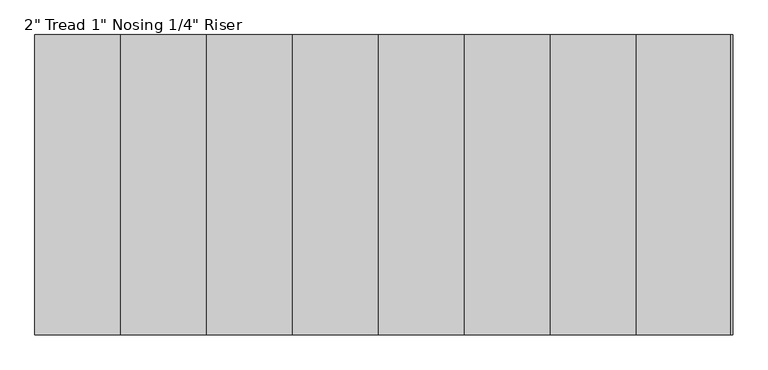
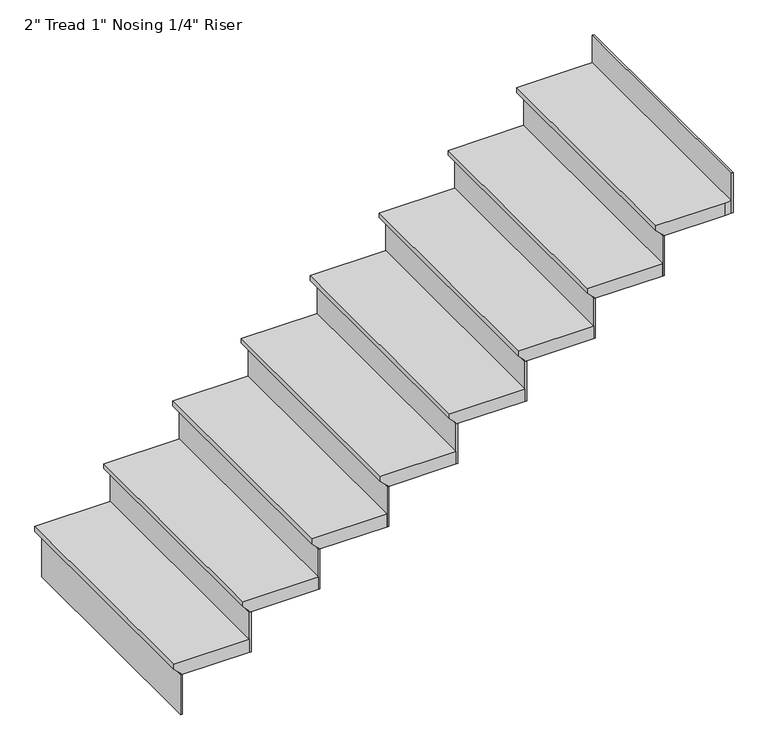
"""IFC4 building model written with IfcOpenShell, lengths in millimetres: stair flight geometry."""

from ifc_helpers import new_model, si_unit, origin, place, context, project, spatial, faceted_brep, source, transform, mapped, element, save


def stair_flight_55fbbb17(model_context):
    return source(origin(), model_context, "Body", "Brep", [
        faceted_brep([(-13886.5772527, 10889.0453953, 943.4763158), (-13886.5772527, 10889.0453953, 962.5263158), (-13886.5772527, 11803.4453953, 962.5263158), (-13886.5772527, 11803.4453953, 943.4763158), (-13861.1772527, 10889.0453953, 918.0763158), (-13861.1772527, 11803.4453953, 918.0763158), (-13599.537409, 10889.0453953, 962.5263158), (-13599.537409, 11803.4453953, 962.5263158), (-13861.1772527, 11803.4453953, 911.7263158), (-13599.537409, 11803.4453953, 911.7263158), (-13599.537409, 10889.0453953, 911.7263158), (-13861.1772527, 10889.0453953, 911.7263158)], [[[0, 1, 2, 3]], [[4, 0, 3, 5]], [[2, 1, 6, 7]], [[8, 9, 10, 11]], [[2, 7, 9, 8, 5, 3]], [[8, 11, 4, 5]], [[6, 1, 0, 4, 11, 10]], [[7, 6, 10, 9]]]),
        faceted_brep([(-13861.1772527, 10889.0453953, 911.7263158), (-13861.1772527, 10889.0453953, 751.3052632), (-13854.8272527, 10889.0453953, 751.3052632), (-13854.8272527, 10889.0453953, 911.7263158), (-13861.1772527, 11803.4453953, 911.7263158), (-13854.8272527, 11803.4453953, 911.7263158), (-13854.8272527, 11803.4453953, 751.3052632), (-13861.1772527, 11803.4453953, 751.3052632)], [[[0, 1, 2, 3]], [[4, 5, 6, 7]], [[1, 0, 4, 7]], [[2, 1, 7, 6]], [[3, 2, 6, 5]], [[0, 3, 5, 4]]]),
        faceted_brep([(-13599.537409, 10889.0453953, 1072.1473684), (-13599.537409, 10889.0453953, 911.7263158), (-13593.187409, 10889.0453953, 911.7263158), (-13593.187409, 10889.0453953, 1072.1473684), (-13599.537409, 11803.4453953, 1072.1473684), (-13593.187409, 11803.4453953, 1072.1473684), (-13593.187409, 11803.4453953, 911.7263158), (-13599.537409, 11803.4453953, 911.7263158)], [[[0, 1, 2, 3]], [[4, 5, 6, 7]], [[1, 0, 4, 7]], [[2, 1, 7, 6]], [[3, 2, 6, 5]], [[0, 3, 5, 4]]]),
        faceted_brep([(-13624.937409, 11803.4453953, 1122.9473684), (-13624.937409, 10889.0453953, 1122.9473684), (-13337.8975652, 10889.0453953, 1122.9473684), (-13337.8975652, 11803.4453953, 1122.9473684), (-13599.537409, 11803.4453953, 1072.1473684), (-13337.8975652, 11803.4453953, 1072.1473684), (-13337.8975652, 10889.0453953, 1072.1473684), (-13599.537409, 10889.0453953, 1072.1473684), (-13599.537409, 11803.4453953, 1078.4973684), (-13624.937409, 11803.4453953, 1103.8973684), (-13599.537409, 10889.0453953, 1078.4973684), (-13624.937409, 10889.0453953, 1103.8973684)], [[[0, 1, 2, 3]], [[4, 5, 6, 7]], [[0, 3, 5, 4, 8, 9]], [[4, 7, 10, 8]], [[2, 1, 11, 10, 7, 6]], [[3, 2, 6, 5]], [[11, 1, 0, 9]], [[10, 11, 9, 8]]]),
        faceted_brep([(-13337.8975652, 10889.0453953, 1232.5684211), (-13337.8975652, 10889.0453953, 1072.1473684), (-13331.5475652, 10889.0453953, 1072.1473684), (-13331.5475652, 10889.0453953, 1232.5684211), (-13337.8975652, 11803.4453953, 1232.5684211), (-13331.5475652, 11803.4453953, 1232.5684211), (-13331.5475652, 11803.4453953, 1072.1473684), (-13337.8975652, 11803.4453953, 1072.1473684)], [[[0, 1, 2, 3]], [[4, 5, 6, 7]], [[1, 0, 4, 7]], [[2, 1, 7, 6]], [[3, 2, 6, 5]], [[0, 3, 5, 4]]]),
        faceted_brep([(-13363.2975652, 11803.4453953, 1283.3684211), (-13363.2975652, 10889.0453953, 1283.3684211), (-13076.2577215, 10889.0453953, 1283.3684211), (-13076.2577215, 11803.4453953, 1283.3684211), (-13337.8975652, 11803.4453953, 1232.5684211), (-13076.2577215, 11803.4453953, 1232.5684211), (-13076.2577215, 10889.0453953, 1232.5684211), (-13337.8975652, 10889.0453953, 1232.5684211), (-13337.8975652, 11803.4453953, 1238.9184211), (-13363.2975652, 11803.4453953, 1264.3184211), (-13337.8975652, 10889.0453953, 1238.9184211), (-13363.2975652, 10889.0453953, 1264.3184211)], [[[0, 1, 2, 3]], [[4, 5, 6, 7]], [[0, 3, 5, 4, 8, 9]], [[4, 7, 10, 8]], [[2, 1, 11, 10, 7, 6]], [[3, 2, 6, 5]], [[11, 1, 0, 9]], [[10, 11, 9, 8]]]),
        faceted_brep([(-13076.2577215, 10889.0453953, 1392.9894737), (-13076.2577215, 10889.0453953, 1232.5684211), (-13069.9077215, 10889.0453953, 1232.5684211), (-13069.9077215, 10889.0453953, 1392.9894737), (-13076.2577215, 11803.4453953, 1392.9894737), (-13069.9077215, 11803.4453953, 1392.9894737), (-13069.9077215, 11803.4453953, 1232.5684211), (-13076.2577215, 11803.4453953, 1232.5684211)], [[[0, 1, 2, 3]], [[4, 5, 6, 7]], [[1, 0, 4, 7]], [[2, 1, 7, 6]], [[3, 2, 6, 5]], [[0, 3, 5, 4]]]),
        faceted_brep([(-13101.6577215, 11803.4453953, 1443.7894737), (-13101.6577215, 10889.0453953, 1443.7894737), (-12814.6178777, 10889.0453953, 1443.7894737), (-12814.6178777, 11803.4453953, 1443.7894737), (-13076.2577215, 11803.4453953, 1392.9894737), (-12814.6178777, 11803.4453953, 1392.9894737), (-12814.6178777, 10889.0453953, 1392.9894737), (-13076.2577215, 10889.0453953, 1392.9894737), (-13076.2577215, 11803.4453953, 1399.3394737), (-13101.6577215, 11803.4453953, 1424.7394737), (-13076.2577215, 10889.0453953, 1399.3394737), (-13101.6577215, 10889.0453953, 1424.7394737)], [[[0, 1, 2, 3]], [[4, 5, 6, 7]], [[0, 3, 5, 4, 8, 9]], [[4, 7, 10, 8]], [[2, 1, 11, 10, 7, 6]], [[3, 2, 6, 5]], [[11, 1, 0, 9]], [[10, 11, 9, 8]]]),
        faceted_brep([(-12814.6178777, 10889.0453953, 1553.4105263), (-12814.6178777, 10889.0453953, 1392.9894737), (-12808.2678777, 10889.0453953, 1392.9894737), (-12808.2678777, 10889.0453953, 1553.4105263), (-12814.6178777, 11803.4453953, 1553.4105263), (-12808.2678777, 11803.4453953, 1553.4105263), (-12808.2678777, 11803.4453953, 1392.9894737), (-12814.6178777, 11803.4453953, 1392.9894737)], [[[0, 1, 2, 3]], [[4, 5, 6, 7]], [[1, 0, 4, 7]], [[2, 1, 7, 6]], [[3, 2, 6, 5]], [[0, 3, 5, 4]]]),
        faceted_brep([(-12840.0178777, 11803.4453953, 1604.2105263), (-12840.0178777, 10889.0453953, 1604.2105263), (-12552.978034, 10889.0453953, 1604.2105263), (-12552.978034, 11803.4453953, 1604.2105263), (-12814.6178777, 11803.4453953, 1553.4105263), (-12552.978034, 11803.4453953, 1553.4105263), (-12552.978034, 10889.0453953, 1553.4105263), (-12814.6178777, 10889.0453953, 1553.4105263), (-12814.6178777, 11803.4453953, 1559.7605263), (-12840.0178777, 11803.4453953, 1585.1605263), (-12814.6178777, 10889.0453953, 1559.7605263), (-12840.0178777, 10889.0453953, 1585.1605263)], [[[0, 1, 2, 3]], [[4, 5, 6, 7]], [[0, 3, 5, 4, 8, 9]], [[4, 7, 10, 8]], [[2, 1, 11, 10, 7, 6]], [[3, 2, 6, 5]], [[11, 1, 0, 9]], [[10, 11, 9, 8]]]),
        faceted_brep([(-12552.978034, 10889.0453953, 1713.8315789), (-12552.978034, 10889.0453953, 1553.4105263), (-12546.628034, 10889.0453953, 1553.4105263), (-12546.628034, 10889.0453953, 1713.8315789), (-12552.978034, 11803.4453953, 1713.8315789), (-12546.628034, 11803.4453953, 1713.8315789), (-12546.628034, 11803.4453953, 1553.4105263), (-12552.978034, 11803.4453953, 1553.4105263)], [[[0, 1, 2, 3]], [[4, 5, 6, 7]], [[1, 0, 4, 7]], [[2, 1, 7, 6]], [[3, 2, 6, 5]], [[0, 3, 5, 4]]]),
        faceted_brep([(-12578.378034, 11803.4453953, 1764.6315789), (-12578.378034, 10889.0453953, 1764.6315789), (-12291.3381902, 10889.0453953, 1764.6315789), (-12291.3381902, 11803.4453953, 1764.6315789), (-12552.978034, 11803.4453953, 1713.8315789), (-12291.3381902, 11803.4453953, 1713.8315789), (-12291.3381902, 10889.0453953, 1713.8315789), (-12552.978034, 10889.0453953, 1713.8315789), (-12552.978034, 11803.4453953, 1720.1815789), (-12578.378034, 11803.4453953, 1745.5815789), (-12552.978034, 10889.0453953, 1720.1815789), (-12578.378034, 10889.0453953, 1745.5815789)], [[[0, 1, 2, 3]], [[4, 5, 6, 7]], [[0, 3, 5, 4, 8, 9]], [[4, 7, 10, 8]], [[2, 1, 11, 10, 7, 6]], [[3, 2, 6, 5]], [[11, 1, 0, 9]], [[10, 11, 9, 8]]]),
        faceted_brep([(-12291.3381902, 10889.0453953, 1874.2526316), (-12291.3381902, 10889.0453953, 1713.8315789), (-12284.9881902, 10889.0453953, 1713.8315789), (-12284.9881902, 10889.0453953, 1874.2526316), (-12291.3381902, 11803.4453953, 1874.2526316), (-12284.9881902, 11803.4453953, 1874.2526316), (-12284.9881902, 11803.4453953, 1713.8315789), (-12291.3381902, 11803.4453953, 1713.8315789)], [[[0, 1, 2, 3]], [[4, 5, 6, 7]], [[1, 0, 4, 7]], [[2, 1, 7, 6]], [[3, 2, 6, 5]], [[0, 3, 5, 4]]]),
        faceted_brep([(-12316.7381902, 11803.4453953, 1925.0526316), (-12316.7381902, 10889.0453953, 1925.0526316), (-12029.6983465, 10889.0453953, 1925.0526316), (-12029.6983465, 11803.4453953, 1925.0526316), (-12291.3381902, 11803.4453953, 1874.2526316), (-12029.6983465, 11803.4453953, 1874.2526316), (-12029.6983465, 10889.0453953, 1874.2526316), (-12291.3381902, 10889.0453953, 1874.2526316), (-12291.3381902, 11803.4453953, 1880.6026316), (-12316.7381902, 11803.4453953, 1906.0026316), (-12291.3381902, 10889.0453953, 1880.6026316), (-12316.7381902, 10889.0453953, 1906.0026316)], [[[0, 1, 2, 3]], [[4, 5, 6, 7]], [[0, 3, 5, 4, 8, 9]], [[4, 7, 10, 8]], [[2, 1, 11, 10, 7, 6]], [[3, 2, 6, 5]], [[11, 1, 0, 9]], [[10, 11, 9, 8]]]),
        faceted_brep([(-11768.0585027, 10889.0453953, 2195.0947368), (-11768.0585027, 10889.0453953, 2034.6736842), (-11761.7085027, 10889.0453953, 2034.6736842), (-11761.7085027, 10889.0453953, 2195.0947368), (-11768.0585027, 11803.4453953, 2195.0947368), (-11761.7085027, 11803.4453953, 2195.0947368), (-11761.7085027, 11803.4453953, 2034.6736842), (-11768.0585027, 11803.4453953, 2034.6736842)], [[[0, 1, 2, 3]], [[4, 5, 6, 7]], [[1, 0, 4, 7]], [[2, 1, 7, 6]], [[3, 2, 6, 5]], [[0, 3, 5, 4]]]),
        faceted_brep([(-12029.6983465, 10889.0453953, 2034.6736842), (-12029.6983465, 10889.0453953, 1874.2526316), (-12023.3483465, 10889.0453953, 1874.2526316), (-12023.3483465, 10889.0453953, 2034.6736842), (-12029.6983465, 11803.4453953, 2034.6736842), (-12023.3483465, 11803.4453953, 2034.6736842), (-12023.3483465, 11803.4453953, 1874.2526316), (-12029.6983465, 11803.4453953, 1874.2526316)], [[[0, 1, 2, 3]], [[4, 5, 6, 7]], [[1, 0, 4, 7]], [[2, 1, 7, 6]], [[3, 2, 6, 5]], [[0, 3, 5, 4]]]),
        faceted_brep([(-11768.0585027, 11803.4453953, 2085.4736842), (-11793.4585027, 11803.4453953, 2085.4736842), (-12055.0983465, 11803.4453953, 2085.4736842), (-12055.0983465, 10889.0453953, 2085.4736842), (-11793.4585027, 10889.0453953, 2085.4736842), (-11768.0585027, 10889.0453953, 2085.4736842), (-11793.4585027, 11803.4453953, 2034.6736842), (-11768.0585027, 11803.4453953, 2034.6736842), (-11768.0585027, 10889.0453953, 2034.6736842), (-11793.4585027, 10889.0453953, 2034.6736842), (-12029.6983465, 10889.0453953, 2034.6736842), (-12029.6983465, 11803.4453953, 2034.6736842), (-12029.6983465, 11803.4453953, 2041.0236842), (-12055.0983465, 11803.4453953, 2066.4236842), (-12029.6983465, 10889.0453953, 2041.0236842), (-12055.0983465, 10889.0453953, 2066.4236842)], [[[0, 1, 2, 3, 4, 5]], [[6, 7, 8, 9, 10, 11]], [[1, 0, 7, 6]], [[2, 1, 6, 11, 12, 13]], [[11, 10, 14, 12]], [[4, 3, 15, 14, 10, 9]], [[5, 4, 9, 8]], [[0, 5, 8, 7]], [[15, 3, 2, 13]], [[14, 15, 13, 12]]]),
    ])


if __name__ == "__main__":
    model = new_model("IFC4")
    model_context = context("Model", 3, world=origin())
    ifc_project = project(units=[si_unit("LENGTHUNIT", "METRE", prefix="MILLI")], contexts=[model_context])
    site = spatial("IfcSite", under=ifc_project)
    building = spatial("IfcBuilding", under=site)
    placement = place(None, origin())
    stair_flight_shape = stair_flight_55fbbb17(model_context)
    element("IfcStairFlight", 1, ObjectType="2\" Tread 1\" Nosing 1/4\" Riser", at=placement, inside=building, context=model_context, shape_type="MappedRepresentation", body=[
        mapped(stair_flight_shape, transform((0.0, 0.0, 0.0), x_axis=(1.0, 0.0, 0.0), y_axis=(0.0, 1.0, 0.0), z_axis=(0.0, 0.0, 1.0))),
    ])
    save(model, "model.ifc")
